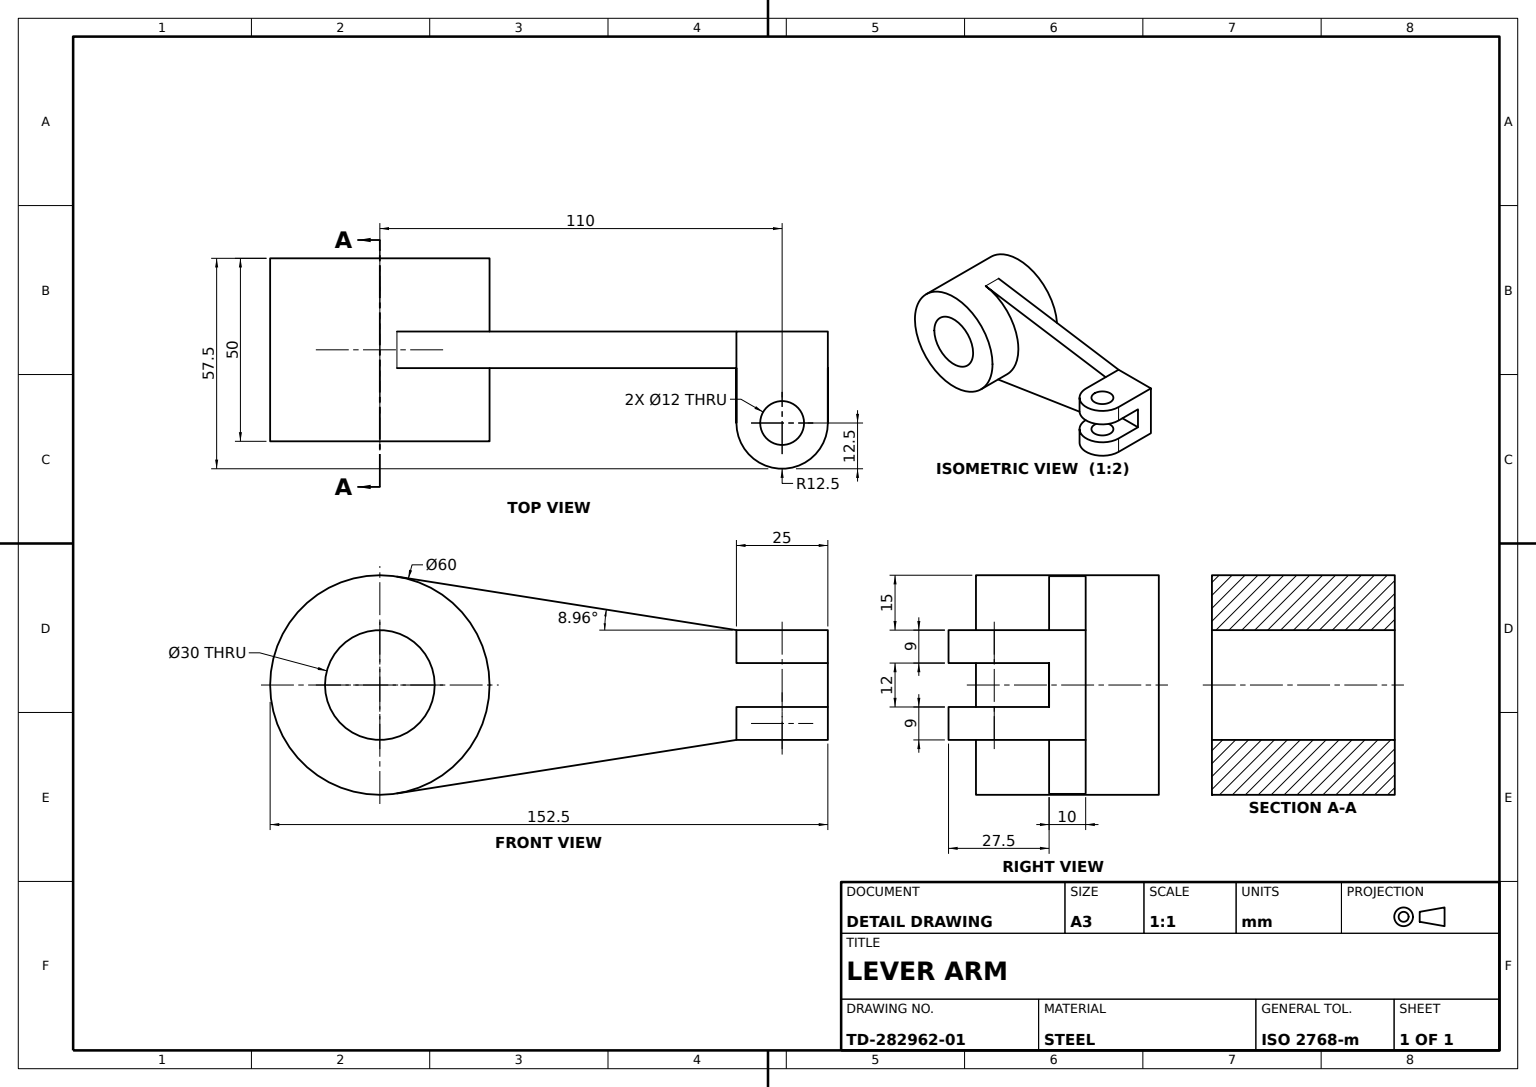
SolidWorks part; units mm, degrees
material "Plain Carbon Steel"
ref_plane "Front Plane" through (0, 0, 0) normal (0, 0, 1) x (1, 0, 0)
ref_plane "Top Plane" through (0, 0, 0) normal (0, 1, 0) x (1, 0, 0)
ref_plane "Right Plane" through (0, 0, 0) normal (1, 0, 0) x (0, 0, -1)
sketch "Hub Profile Sketch" plane through (0, 0, 0) normal (0, 0, 1) x (1, 0, 0)
  line L0 (0, 58.5113) -> (0, -50.5626) construction
  line L1 (-81.695, 0) -> (63.5896, 0) construction
  circle A0 centre (0, 0) radius 15
  circle A1 centre (0, 0) radius 30
  dimension "D1" = 60
  dimension "D2" = 30
extrude "Hub Ø60 Bore Ø30" add sketch "Hub Profile Sketch" along normal mid plane 50
sketch "Lever Arm Sketch" plane through (0, 0, 0) normal (0, 0, 1) x (1, 0, 0)
  line L0 (-50.4775, 0) -> (138.088, 0) construction
  line L1 (4.6717, 29.634) -> (97.5, 15)
  line L2 (97.5, 15) -> (122.5, 15)
  line L3 (122.5, 15) -> (122.5, -15)
  line L4 (97.5, -15) -> (122.5, -15)
  line L5 (4.6717, -29.634) -> (97.5, -15)
  circle A1 centre (0, 0) radius 30 construction
  arc A2 (4.6717, -29.634) -> (4.6717, 29.634) centre (0, 0) ccw
  point P10 (110, 15)
  point P12 (122.5, 0)
  dimension "D1" = 15
  dimension "D2" = 25
  dimension "D3" = 110
extrude "Lever Arm Web" add sketch "Lever Arm Sketch" along normal mid plane 10
sketch "Clevis Lug Sketch" plane through (0, -15, 0) normal (0, -1, 0) x (1, 0, 0)
  line L0 (110, 22.6299) -> (110, -17.0595) construction
  line L1 (97.5, -5) -> (122.5, -5) construction
  line L2 (97.5, 5) -> (97.5, 20)
  line L3 (122.5, 5) -> (122.5, 20)
  line L4 (97.5, 5) -> (122.5, 5)
  arc A0 (122.5, 20) -> (97.5, 20) centre (110, 20) ccw
  circle A1 centre (110, 20) radius 6
  dimension "D2" = 25
  dimension "D3" = 12
  dimension "D1" = 110
  dimension "D4" = 25
extrude "Clevis Lug" add sketch "Clevis Lug Sketch" against normal blind 9
mirror "Clevis Lug Mirror" about plane through (0, 0, 0) normal (0, 1, 0) of "Clevis Lug"
